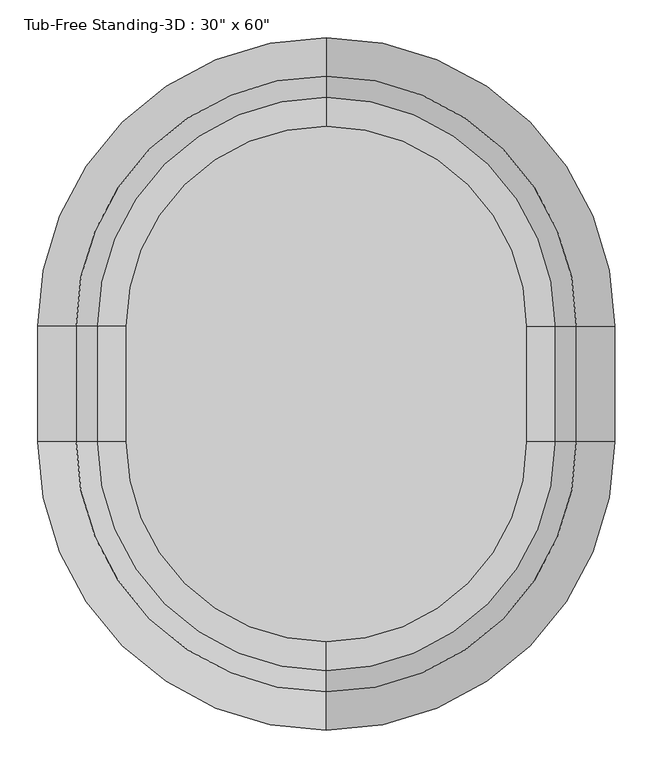
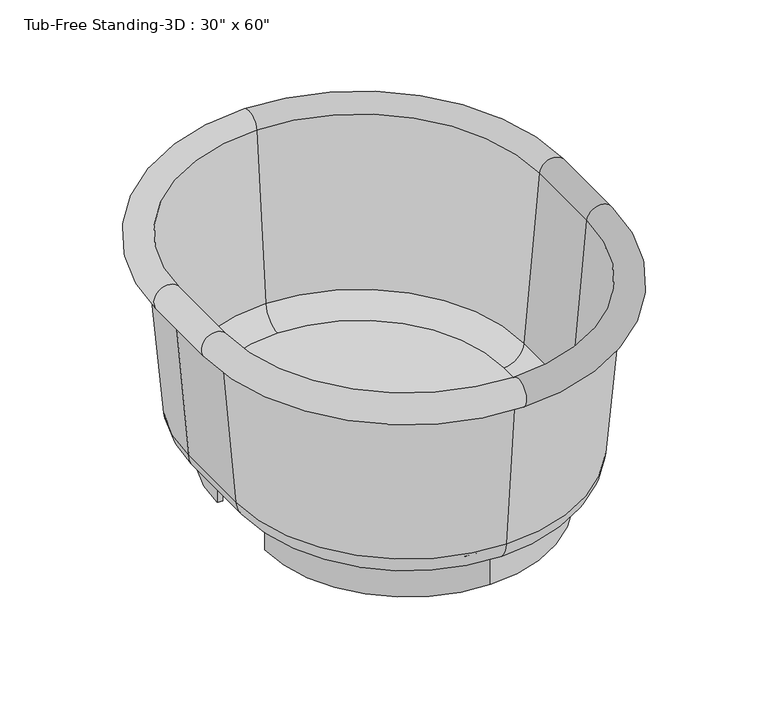
"""IFC4 building model written with IfcOpenShell, lengths in millimetres: flow terminal geometry."""

from ifc_helpers import new_model, si_unit, point, frame, frame_2d, origin, origin_with_axes, place, context, project, spatial, polyline, circle_curve, ellipse_curve, trimmed, segment, composite_curve, outline, extrude, source, transform, mapped, element, save
from ifc_brep_helpers import plane_surface, cylinder_surface, revolved_surface, advanced_brep


def flow_terminal_2ca5ee5d(model_context):
    return source(origin(), model_context, "Body", "SolidModel", [
        extrude(outline(composite_curve([segment(trimmed(circle_curve(frame_2d((0.0, 76.2)), 254.0), [point((0.0, 330.2))], [point((-254.0, 76.2))], True, "CARTESIAN"), True, "CONTINUOUS"), segment(polyline([(-254.0, 76.2), (-264.2824236, 76.2)]), True, "CONTINUOUS"), segment(trimmed(circle_curve(frame_2d((0.0, 76.2)), 264.2824236), [point((-264.2824236, 76.2))], [point((0.0, 340.4824236))], False, "CARTESIAN"), True, "CONTINUOUS"), segment(trimmed(circle_curve(frame_2d((0.0, 76.2)), 264.2824236), [point((0.0, 340.4824236))], [point((264.2824236, 76.2))], False, "CARTESIAN"), True, "CONTINUOUS"), segment(polyline([(264.2824236, 76.2), (254.0, 76.2)]), True, "CONTINUOUS"), segment(trimmed(circle_curve(frame_2d((0.0, 76.2)), 254.0), [point((254.0, 76.2))], [point((0.0, 330.2))], True, "CARTESIAN"), True, "CONTINUOUS")], self_intersect=False)), origin_with_axes(), (0.0, 0.0, 1.0), 63.5),
        extrude(outline(composite_curve([segment(trimmed(circle_curve(frame_2d((0.0, -76.2)), 264.2824236), [point((0.0, -340.4824236))], [point((-264.2824236, -76.2))], False, "CARTESIAN"), True, "CONTINUOUS"), segment(polyline([(-264.2824236, -76.2), (-254.0, -76.2)]), True, "CONTINUOUS"), segment(trimmed(circle_curve(frame_2d((0.0, -76.2)), 254.0), [point((-254.0, -76.2))], [point((0.0, -330.2))], True, "CARTESIAN"), True, "CONTINUOUS"), segment(trimmed(circle_curve(frame_2d((0.0, -76.2)), 254.0), [point((0.0, -330.2))], [point((254.0, -76.2))], True, "CARTESIAN"), True, "CONTINUOUS"), segment(polyline([(254.0, -76.2), (264.2824236, -76.2)]), True, "CONTINUOUS"), segment(trimmed(circle_curve(frame_2d((0.0, -76.2)), 264.2824236), [point((264.2824236, -76.2))], [point((0.0, -340.4824236))], False, "CARTESIAN"), True, "CONTINUOUS")], self_intersect=False)), origin_with_axes(), (0.0, 0.0, 1.0), 63.5),
        extrude(outline(composite_curve([segment(polyline([(-264.2824236, -76.2), (-264.2824236, 76.2)]), True, "CONTINUOUS"), segment(trimmed(circle_curve(frame_2d((0.0, 76.2)), 264.2824236), [point((-264.2824236, 76.2))], [point((0.0, 340.4824236))], False, "CARTESIAN"), True, "CONTINUOUS"), segment(trimmed(circle_curve(frame_2d((0.0, 76.2)), 264.2824236), [point((0.0, 340.4824236))], [point((264.2824236, 76.2))], False, "CARTESIAN"), True, "CONTINUOUS"), segment(polyline([(264.2824236, 76.2), (264.2824236, -76.2)]), True, "CONTINUOUS"), segment(trimmed(circle_curve(frame_2d((0.0, -76.2)), 264.2824236), [point((264.2824236, -76.2))], [point((0.0, -340.4824236))], False, "CARTESIAN"), True, "CONTINUOUS"), segment(trimmed(circle_curve(frame_2d((0.0, -76.2)), 264.2824236), [point((0.0, -340.4824236))], [point((-264.2824236, -76.2))], False, "CARTESIAN"), True, "CONTINUOUS")], self_intersect=False)), frame((0.0, 0.0, 63.5), z_axis=(0.0, 0.0, 1.0), x_axis=(1.0, 0.0, 0.0)), (0.0, 0.0, 1.0), 15.08125),
        advanced_brep(
        [(0.0, -419.1, 406.4), (342.9, -76.2, 406.4), (355.6, -76.2, 406.4), (0.0, -431.8, 406.4), (0.0, -393.3045038, 111.5561295), (317.1045038, -76.2, 111.5561295), (0.0, -340.4824236, 63.1536107), (264.2824236, -76.2, 63.1536107), (0.0, -340.4824236, 78.0774627), (264.2824236, -76.2, 78.0774627), (0.0, -378.4374416, 112.8568289), (302.2374416, -76.2, 112.8568289), (0.0, -406.6561556, 435.3982063), (330.4561556, -76.2, 435.3982063), (-342.9, -76.2, 406.4), (-355.6, -76.2, 406.4), (-317.1045038, -76.2, 111.5561295), (-264.2824236, -76.2, 63.1536107), (-264.2824236, -76.2, 78.0774627), (-302.2374416, -76.2, 112.8568289), (-330.4561556, -76.2, 435.3982063), (-355.6, 76.2, 406.4), (-342.9, 76.2, 406.4), (-317.1045038, 76.2, 111.5561295), (-264.2824236, 76.2, 63.1536107), (-264.2824236, 76.2, 78.0774627), (-302.2374416, 76.2, 112.8568289), (-330.4561556, 76.2, 435.3982063), (0.0, 419.1, 406.4), (0.0, 431.8, 406.4), (0.0, 393.3045038, 111.5561295), (0.0, 340.4824236, 63.1536107), (0.0, 340.4824236, 78.0774627), (0.0, 378.4374416, 112.8568289), (0.0, 406.6561556, 435.3982063), (342.9, 76.2, 406.4), (355.6, 76.2, 406.4), (317.1045038, 76.2, 111.5561295), (264.2824236, 76.2, 63.1536107), (264.2824236, 76.2, 78.0774627), (302.2374416, 76.2, 112.8568289), (330.4561556, 76.2, 435.3982063)],
        [
            (0, 1, circle_curve(frame((0.0, -76.2, 406.4), z_axis=(0.0, 0.0, 1.0), x_axis=(1.0, 0.0, 0.0)), 342.9)),
            (1, 2),
            (2, 3, circle_curve(frame((0.0, -76.2, 406.4), z_axis=(0.0, 0.0, -1.0), x_axis=(1.0, 0.0, 0.0)), 355.6)),
            (3, 0),
            (4, 5, circle_curve(frame((0.0, -76.2, 111.5561295), z_axis=(0.0, 0.0, 1.0), x_axis=(1.0, 0.0, 0.0)), 317.1045038)),
            (5, 1),
            (0, 4),
            (6, 7, circle_curve(frame((0.0, -76.2, 63.1536107), z_axis=(0.0, 0.0, 1.0), x_axis=(1.0, 0.0, 0.0)), 264.2824236)),
            (7, 5, circle_curve(frame((264.2824236, -76.2, 116.1774627), z_axis=(0.0, -1.0, 0.0), x_axis=(1.0, 0.0, 0.0)), 53.023852)),
            (4, 6, circle_curve(frame((0.0, -340.4824236, 116.1774627), z_axis=(1.0, 0.0, 0.0), x_axis=(0.0, -1.0, 0.0)), 53.023852)),
            (8, 9, circle_curve(frame((0.0, -76.2, 78.0774627), z_axis=(0.0, 0.0, 1.0), x_axis=(1.0, 0.0, 0.0)), 264.2824236)),
            (9, 7),
            (6, 8),
            (10, 11, circle_curve(frame((0.0, -76.2, 112.8568289), z_axis=(0.0, 0.0, 1.0), x_axis=(1.0, 0.0, 0.0)), 302.2374416)),
            (11, 9, circle_curve(frame((264.2824236, -76.2, 116.1774627), z_axis=(0.0, 1.0, 0.0), x_axis=(1.0, 0.0, 0.0)), 38.1)),
            (8, 10, circle_curve(frame((0.0, -340.4824236, 116.1774627), z_axis=(-1.0, 0.0, 0.0), x_axis=(0.0, -1.0, 0.0)), 38.1)),
            (12, 13, circle_curve(frame((0.0, -76.2, 435.3982063), z_axis=(0.0, 0.0, 1.0), x_axis=(1.0, 0.0, 0.0)), 330.4561556)),
            (13, 11),
            (10, 12),
            (2, 13, circle_curve(frame((355.6, -76.2, 431.8), z_axis=(0.0, -1.0, 0.0), x_axis=(1.0, 0.0, 0.0)), 25.4)),
            (12, 3, circle_curve(frame((0.0, -431.8, 431.8), z_axis=(1.0, 0.0, 0.0), x_axis=(0.0, -1.0, 0.0)), 25.4)),
            (14, 0, circle_curve(frame((0.0, -76.2, 406.4), z_axis=(0.0, 0.0, 1.0), x_axis=(0.0, -1.0, 0.0)), 342.9)),
            (3, 15, circle_curve(frame((0.0, -76.2, 406.4), z_axis=(0.0, 0.0, -1.0), x_axis=(0.0, -1.0, 0.0)), 355.6)),
            (15, 14),
            (16, 4, circle_curve(frame((0.0, -76.2, 111.5561295), z_axis=(0.0, 0.0, 1.0), x_axis=(0.0, -1.0, 0.0)), 317.1045038)),
            (14, 16),
            (17, 6, circle_curve(frame((0.0, -76.2, 63.1536107), z_axis=(0.0, 0.0, 1.0), x_axis=(0.0, -1.0, 0.0)), 264.2824236)),
            (16, 17, circle_curve(frame((-264.2824236, -76.2, 116.1774627), z_axis=(0.0, -1.0, 0.0), x_axis=(-1.0, 0.0, 0.0)), 53.023852)),
            (18, 8, circle_curve(frame((0.0, -76.2, 78.0774627), z_axis=(0.0, 0.0, 1.0), x_axis=(0.0, -1.0, 0.0)), 264.2824236)),
            (17, 18),
            (19, 10, circle_curve(frame((0.0, -76.2, 112.8568289), z_axis=(0.0, 0.0, 1.0), x_axis=(0.0, -1.0, 0.0)), 302.2374416)),
            (18, 19, circle_curve(frame((-264.2824236, -76.2, 116.1774627), z_axis=(0.0, 1.0, 0.0), x_axis=(-1.0, 0.0, 0.0)), 38.1)),
            (20, 12, circle_curve(frame((0.0, -76.2, 435.3982063), z_axis=(0.0, 0.0, 1.0), x_axis=(0.0, -1.0, 0.0)), 330.4561556)),
            (19, 20),
            (20, 15, circle_curve(frame((-355.6, -76.2, 431.8), z_axis=(0.0, -1.0, 0.0), x_axis=(-1.0, 0.0, 0.0)), 25.4)),
            (15, 21),
            (21, 22),
            (22, 14),
            (22, 23),
            (23, 16),
            (23, 24, circle_curve(frame((-264.2824236, 76.2, 116.1774627), z_axis=(0.0, -1.0, 0.0), x_axis=(-1.0, 0.0, 0.0)), 53.023852)),
            (24, 17),
            (24, 25),
            (25, 18),
            (25, 26, circle_curve(frame((-264.2824236, 76.2, 116.1774627), z_axis=(0.0, 1.0, 0.0), x_axis=(-1.0, 0.0, 0.0)), 38.1)),
            (26, 19),
            (26, 27),
            (27, 20),
            (27, 21, circle_curve(frame((-355.6, 76.2, 431.8), z_axis=(0.0, -1.0, 0.0), x_axis=(-1.0, 0.0, 0.0)), 25.4)),
            (28, 22, circle_curve(frame((0.0, 76.2, 406.4), z_axis=(0.0, 0.0, 1.0), x_axis=(-1.0, 0.0, 0.0)), 342.9)),
            (21, 29, circle_curve(frame((0.0, 76.2, 406.4), z_axis=(0.0, 0.0, -1.0), x_axis=(-1.0, 0.0, 0.0)), 355.6)),
            (29, 28),
            (30, 23, circle_curve(frame((0.0, 76.2, 111.5561295), z_axis=(0.0, 0.0, 1.0), x_axis=(-1.0, 0.0, 0.0)), 317.1045038)),
            (28, 30),
            (31, 24, circle_curve(frame((0.0, 76.2, 63.1536107), z_axis=(0.0, 0.0, 1.0), x_axis=(-1.0, 0.0, 0.0)), 264.2824236)),
            (30, 31, circle_curve(frame((0.0, 340.4824236, 116.1774627), z_axis=(-1.0, 0.0, 0.0), x_axis=(0.0, 1.0, 0.0)), 53.023852)),
            (32, 25, circle_curve(frame((0.0, 76.2, 78.0774627), z_axis=(0.0, 0.0, 1.0), x_axis=(-1.0, 0.0, 0.0)), 264.2824236)),
            (31, 32),
            (33, 26, circle_curve(frame((0.0, 76.2, 112.8568289), z_axis=(0.0, 0.0, 1.0), x_axis=(-1.0, 0.0, 0.0)), 302.2374416)),
            (32, 33, circle_curve(frame((0.0, 340.4824236, 116.1774627), z_axis=(1.0, 0.0, 0.0), x_axis=(0.0, 1.0, 0.0)), 38.1)),
            (34, 27, circle_curve(frame((0.0, 76.2, 435.3982063), z_axis=(0.0, 0.0, 1.0), x_axis=(-1.0, 0.0, 0.0)), 330.4561556)),
            (33, 34),
            (34, 29, circle_curve(frame((0.0, 431.8, 431.8), z_axis=(-1.0, 0.0, 0.0), x_axis=(0.0, 1.0, 0.0)), 25.4)),
            (35, 28, circle_curve(frame((0.0, 76.2, 406.4), z_axis=(0.0, 0.0, 1.0), x_axis=(0.0, 1.0, 0.0)), 342.9)),
            (29, 36, circle_curve(frame((0.0, 76.2, 406.4), z_axis=(0.0, 0.0, -1.0), x_axis=(0.0, 1.0, 0.0)), 355.6)),
            (36, 35),
            (37, 30, circle_curve(frame((0.0, 76.2, 111.5561295), z_axis=(0.0, 0.0, 1.0), x_axis=(0.0, 1.0, 0.0)), 317.1045038)),
            (35, 37),
            (38, 31, circle_curve(frame((0.0, 76.2, 63.1536107), z_axis=(0.0, 0.0, 1.0), x_axis=(0.0, 1.0, 0.0)), 264.2824236)),
            (37, 38, circle_curve(frame((264.2824236, 76.2, 116.1774627), z_axis=(0.0, 1.0, 0.0), x_axis=(1.0, 0.0, 0.0)), 53.023852)),
            (39, 32, circle_curve(frame((0.0, 76.2, 78.0774627), z_axis=(0.0, 0.0, 1.0), x_axis=(0.0, 1.0, 0.0)), 264.2824236)),
            (38, 39),
            (40, 33, circle_curve(frame((0.0, 76.2, 112.8568289), z_axis=(0.0, 0.0, 1.0), x_axis=(0.0, 1.0, 0.0)), 302.2374416)),
            (39, 40, circle_curve(frame((264.2824236, 76.2, 116.1774627), z_axis=(0.0, -1.0, 0.0), x_axis=(1.0, 0.0, 0.0)), 38.1)),
            (41, 34, circle_curve(frame((0.0, 76.2, 435.3982063), z_axis=(0.0, 0.0, 1.0), x_axis=(0.0, 1.0, 0.0)), 330.4561556)),
            (40, 41),
            (41, 36, circle_curve(frame((355.6, 76.2, 431.8), z_axis=(0.0, 1.0, 0.0), x_axis=(1.0, 0.0, 0.0)), 25.4)),
            (36, 2),
            (1, 35),
            (5, 37),
            (7, 38),
            (9, 39),
            (11, 40),
            (13, 41),
        ],
        [
            plane_surface(frame((0.0, -76.2, 406.4), z_axis=(0.0, 0.0, -1.0), x_axis=(1.0, 0.0, 0.0))),
            revolved_surface(polyline([(342.9, -76.2, 406.4), (317.1045038, -76.2, 111.5561295)]), (0.0, -76.2, 431.8), (0.0, 0.0, -1.0)),
            revolved_surface(trimmed(ellipse_curve(frame((264.2824236, -76.2, 116.1774627), z_axis=(0.0, 1.0, 0.0), x_axis=(1.0, 0.0, 0.0)), 53.023852, 53.023852), [point((317.1045038, -76.2, 111.5561295))], [point((264.2824236, -76.2, 63.1536107))], True, "CARTESIAN"), (0.0, -76.2, 431.8), (0.0, 0.0, -1.0)),
            revolved_surface(polyline([(264.2824236, -76.2, 63.1536107), (264.2824236, -76.2, 78.07746270000001)]), (0.0, -76.2, 431.8), (0.0, 0.0, -1.0)),
            revolved_surface(trimmed(ellipse_curve(frame((264.2824236, -76.2, 116.1774627), z_axis=(0.0, -1.0, 0.0), x_axis=(1.0, 0.0, 0.0)), 38.1, 38.1), [point((264.2824236, -76.2, 78.0774627))], [point((302.2374416, -76.2, 112.8568289))], True, "CARTESIAN"), (0.0, -76.2, 431.8), (0.0, 0.0, -1.0)),
            revolved_surface(polyline([(302.2374416, -76.2, 112.8568289), (330.4561556, -76.2, 435.3982063)]), (0.0, -76.2, 431.8), (0.0, 0.0, -1.0)),
            revolved_surface(trimmed(ellipse_curve(frame((355.6, -76.2, 431.8), z_axis=(0.0, 1.0, 0.0), x_axis=(1.0, 0.0, 0.0)), 25.4, 25.4), [point((330.4561556, -76.2, 435.3982063))], [point((355.6, -76.2, 406.4))], True, "CARTESIAN"), (0.0, -76.2, 431.8), (0.0, 0.0, -1.0)),
            plane_surface(frame((0.0, -76.2, 406.4), z_axis=(0.0, 0.0, -1.0), x_axis=(0.0, -1.0, 0.0))),
            revolved_surface(polyline([(0.0, -419.1, 406.4), (0.0, -393.3045038, 111.5561295)]), (0.0, -76.2, 431.8), (0.0, 0.0, -1.0)),
            revolved_surface(trimmed(ellipse_curve(frame((0.0, -340.4824236, 116.1774627), z_axis=(1.0, 0.0, 0.0), x_axis=(0.0, -1.0, 0.0)), 53.023852, 53.023852), [point((0.0, -393.3045038, 111.5561295))], [point((0.0, -340.4824236, 63.1536107))], True, "CARTESIAN"), (0.0, -76.2, 431.8), (0.0, 0.0, -1.0)),
            revolved_surface(polyline([(0.0, -340.4824236, 63.1536107), (0.0, -340.4824236, 78.07746270000001)]), (0.0, -76.2, 431.8), (0.0, 0.0, -1.0)),
            revolved_surface(trimmed(ellipse_curve(frame((0.0, -340.4824236, 116.1774627), z_axis=(-1.0, 0.0, 0.0), x_axis=(0.0, -1.0, 0.0)), 38.1, 38.1), [point((0.0, -340.4824236, 78.0774627))], [point((0.0, -378.4374416, 112.8568289))], True, "CARTESIAN"), (0.0, -76.2, 431.8), (0.0, 0.0, -1.0)),
            revolved_surface(polyline([(0.0, -378.4374416, 112.8568289), (0.0, -406.6561556, 435.3982063)]), (0.0, -76.2, 431.8), (0.0, 0.0, -1.0)),
            revolved_surface(trimmed(ellipse_curve(frame((0.0, -431.8, 431.8), z_axis=(1.0, 0.0, 0.0), x_axis=(0.0, -1.0, 0.0)), 25.4, 25.4), [point((0.0, -406.6561556, 435.3982063))], [point((0.0, -431.8, 406.4))], True, "CARTESIAN"), (0.0, -76.2, 431.8), (0.0, 0.0, -1.0)),
            plane_surface(frame((-355.6, -76.2, 406.4), z_axis=(0.0, 0.0, -1.0), x_axis=(0.0, 1.0, 0.0))),
            plane_surface(frame((-342.9, -76.2, 406.4), z_axis=(-0.9961946980917455, 0.0, -0.08715574274765871), x_axis=(0.0, 1.0, 0.0))),
            cylinder_surface(frame((-264.2824236, -76.2, 116.1774627), z_axis=(0.0, -1.0, 0.0), x_axis=(-1.0, 0.0, 0.0)), 53.023852),
            plane_surface(frame((-264.2824236, -76.2, 63.1536107), z_axis=(1.0, 0.0, 0.0), x_axis=(0.0, 1.0, 0.0))),
            revolved_surface(polyline([(-302.38242360000004, 76.2, 116.1774627), (-302.38242360000004, -76.2, 116.1774627)]), (-264.2824236, -76.2, 116.1774627), (0.0, 1.0, 0.0)),
            plane_surface(frame((-302.2374416, -76.2, 112.8568289), z_axis=(0.9961946980917458, 0.0, 0.08715574274765651), x_axis=(0.0, 1.0, 0.0))),
            cylinder_surface(frame((-355.6, -76.2, 431.8), z_axis=(0.0, -1.0, 0.0), x_axis=(-1.0, 0.0, 0.0)), 25.4),
            plane_surface(frame((0.0, 76.2, 406.4), z_axis=(0.0, 0.0, -1.0), x_axis=(-1.0, 0.0, 0.0))),
            revolved_surface(polyline([(-342.9, 76.2, 406.4), (-317.1045038, 76.2, 111.5561295)]), (0.0, 76.2, 431.8), (0.0, 0.0, -1.0)),
            revolved_surface(trimmed(ellipse_curve(frame((-264.2824236, 76.2, 116.1774627), z_axis=(0.0, -1.0, 0.0), x_axis=(-1.0, 0.0, 0.0)), 53.023852, 53.023852), [point((-317.1045038, 76.2, 111.5561295))], [point((-264.2824236, 76.2, 63.1536107))], True, "CARTESIAN"), (0.0, 76.2, 431.8), (0.0, 0.0, -1.0)),
            revolved_surface(polyline([(-264.2824236, 76.2, 63.1536107), (-264.2824236, 76.2, 78.07746270000001)]), (0.0, 76.2, 431.8), (0.0, 0.0, -1.0)),
            revolved_surface(trimmed(ellipse_curve(frame((-264.2824236, 76.2, 116.1774627), z_axis=(0.0, 1.0, 0.0), x_axis=(-1.0, 0.0, 0.0)), 38.1, 38.1), [point((-264.2824236, 76.2, 78.0774627))], [point((-302.2374416, 76.2, 112.8568289))], True, "CARTESIAN"), (0.0, 76.2, 431.8), (0.0, 0.0, -1.0)),
            revolved_surface(polyline([(-302.2374416, 76.2, 112.8568289), (-330.4561556, 76.2, 435.3982063)]), (0.0, 76.2, 431.8), (0.0, 0.0, -1.0)),
            revolved_surface(trimmed(ellipse_curve(frame((-355.6, 76.2, 431.8), z_axis=(0.0, -1.0, 0.0), x_axis=(-1.0, 0.0, 0.0)), 25.4, 25.4), [point((-330.4561556, 76.2, 435.3982063))], [point((-355.6, 76.2, 406.4))], True, "CARTESIAN"), (0.0, 76.2, 431.8), (0.0, 0.0, -1.0)),
            plane_surface(frame((0.0, 76.2, 406.4), z_axis=(0.0, 0.0, -1.0), x_axis=(0.0, 1.0, 0.0))),
            revolved_surface(polyline([(0.0, 419.1, 406.4), (0.0, 393.3045038, 111.5561295)]), (0.0, 76.2, 431.8), (0.0, 0.0, -1.0)),
            revolved_surface(trimmed(ellipse_curve(frame((0.0, 340.4824236, 116.1774627), z_axis=(-1.0, 0.0, 0.0), x_axis=(0.0, 1.0, 0.0)), 53.023852, 53.023852), [point((0.0, 393.3045038, 111.5561295))], [point((0.0, 340.4824236, 63.1536107))], True, "CARTESIAN"), (0.0, 76.2, 431.8), (0.0, 0.0, -1.0)),
            revolved_surface(polyline([(0.0, 340.4824236, 63.1536107), (0.0, 340.4824236, 78.07746270000001)]), (0.0, 76.2, 431.8), (0.0, 0.0, -1.0)),
            revolved_surface(trimmed(ellipse_curve(frame((0.0, 340.4824236, 116.1774627), z_axis=(1.0, 0.0, 0.0), x_axis=(0.0, 1.0, 0.0)), 38.1, 38.1), [point((0.0, 340.4824236, 78.0774627))], [point((0.0, 378.4374416, 112.8568289))], True, "CARTESIAN"), (0.0, 76.2, 431.8), (0.0, 0.0, -1.0)),
            revolved_surface(polyline([(0.0, 378.4374416, 112.8568289), (0.0, 406.6561556, 435.3982063)]), (0.0, 76.2, 431.8), (0.0, 0.0, -1.0)),
            revolved_surface(trimmed(ellipse_curve(frame((0.0, 431.8, 431.8), z_axis=(-1.0, 0.0, 0.0), x_axis=(0.0, 1.0, 0.0)), 25.4, 25.4), [point((0.0, 406.6561556, 435.3982063))], [point((0.0, 431.8, 406.4))], True, "CARTESIAN"), (0.0, 76.2, 431.8), (0.0, 0.0, -1.0)),
            plane_surface(frame((355.6, 76.2, 406.4), z_axis=(0.0, 0.0, -1.0), x_axis=(0.0, -1.0, 0.0))),
            plane_surface(frame((342.9, 76.2, 406.4), z_axis=(0.9961946980917455, 0.0, -0.08715574274765871), x_axis=(0.0, -1.0, 0.0))),
            cylinder_surface(frame((264.2824236, 76.2, 116.1774627), z_axis=(0.0, 1.0, 0.0), x_axis=(1.0, 0.0, 0.0)), 53.023852),
            plane_surface(frame((264.2824236, 76.2, 63.1536107), z_axis=(-1.0, 0.0, 0.0), x_axis=(0.0, -1.0, 0.0))),
            revolved_surface(polyline([(302.38242360000004, -76.2, 116.1774627), (302.38242360000004, 76.2, 116.1774627)]), (264.2824236, 76.2, 116.1774627), (0.0, -1.0, 0.0)),
            plane_surface(frame((302.2374416, 76.2, 112.8568289), z_axis=(-0.9961946980917458, 0.0, 0.08715574274765651), x_axis=(0.0, -1.0, 0.0))),
            cylinder_surface(frame((355.6, 76.2, 431.8), z_axis=(0.0, 1.0, 0.0), x_axis=(1.0, 0.0, 0.0)), 25.4),
        ],
        [
            (0, [[1, 2, 3, 4]]),
            (1, [[5, 6, -1, 7]]),
            (2, [[8, 9, -5, 10]]),
            (3, [[11, 12, -8, 13]]),
            (4, [[14, 15, -11, 16]]),
            (5, [[17, 18, -14, 19]]),
            (6, [[-3, 20, -17, 21]]),
            (7, [[22, -4, 23, 24]]),
            (8, [[25, -7, -22, 26]]),
            (9, [[27, -10, -25, 28]]),
            (10, [[29, -13, -27, 30]]),
            (11, [[31, -16, -29, 32]]),
            (12, [[33, -19, -31, 34]]),
            (13, [[-23, -21, -33, 35]]),
            (14, [[-24, 36, 37, 38]]),
            (15, [[-26, -38, 39, 40]]),
            (16, [[-28, -40, 41, 42]]),
            (17, [[-30, -42, 43, 44]]),
            (18, [[-32, -44, 45, 46]]),
            (19, [[-34, -46, 47, 48]]),
            (20, [[-35, -48, 49, -36]]),
            (21, [[50, -37, 51, 52]]),
            (22, [[53, -39, -50, 54]]),
            (23, [[55, -41, -53, 56]]),
            (24, [[57, -43, -55, 58]]),
            (25, [[59, -45, -57, 60]]),
            (26, [[61, -47, -59, 62]]),
            (27, [[-51, -49, -61, 63]]),
            (28, [[64, -52, 65, 66]]),
            (29, [[67, -54, -64, 68]]),
            (30, [[69, -56, -67, 70]]),
            (31, [[71, -58, -69, 72]]),
            (32, [[73, -60, -71, 74]]),
            (33, [[75, -62, -73, 76]]),
            (34, [[-65, -63, -75, 77]]),
            (35, [[-66, 78, -2, 79]]),
            (36, [[-68, -79, -6, 80]]),
            (37, [[-70, -80, -9, 81]]),
            (38, [[-72, -81, -12, 82]]),
            (39, [[-74, -82, -15, 83]]),
            (40, [[-76, -83, -18, 84]]),
            (41, [[-77, -84, -20, -78]]),
        ],
    ),
    ])


if __name__ == "__main__":
    model = new_model("IFC4")
    model_context = context("Model", 3, world=origin())
    ifc_project = project(units=[si_unit("LENGTHUNIT", "METRE", prefix="MILLI")], contexts=[model_context])
    site = spatial("IfcSite", under=ifc_project)
    building = spatial("IfcBuilding", under=site)
    placement = place(None, origin())
    flow_terminal_shape = flow_terminal_2ca5ee5d(model_context)
    element("IfcFlowTerminal", 1, ObjectType="Tub-Free Standing-3D : 30\" x 60\"", at=placement, inside=building, context=model_context, shape_type="MappedRepresentation", body=[
        mapped(flow_terminal_shape, transform((0.0, 0.0, 0.0), x_axis=(1.0, 0.0, 0.0), y_axis=(0.0, 1.0, 0.0), z_axis=(0.0, 0.0, 1.0))),
    ])
    save(model, "model.ifc")

# Revit data of these elements
# Type "Tub-Free Standing-3D : 30\" x 60\""
#   Assembly Code = "D2010110"
#   Height = 1' - 6"
#   Length = 3' - 0"
#   Width = 2' - 6"
#   Tub Material = Porcelain, Ivory
#   Default Elevation = 0
# Element 1 (IfcFlowTerminal, "Tub-Free Standing-3D : 30\" x 60\"")
#   Materials on its faces: "Porcelain, Ivory"
# Materials
#   "Porcelain, Ivory": class "Ceramic", colour RGB 247 247 239, transparency 0, Description = "Porcelain, ivory", Cost = 0
